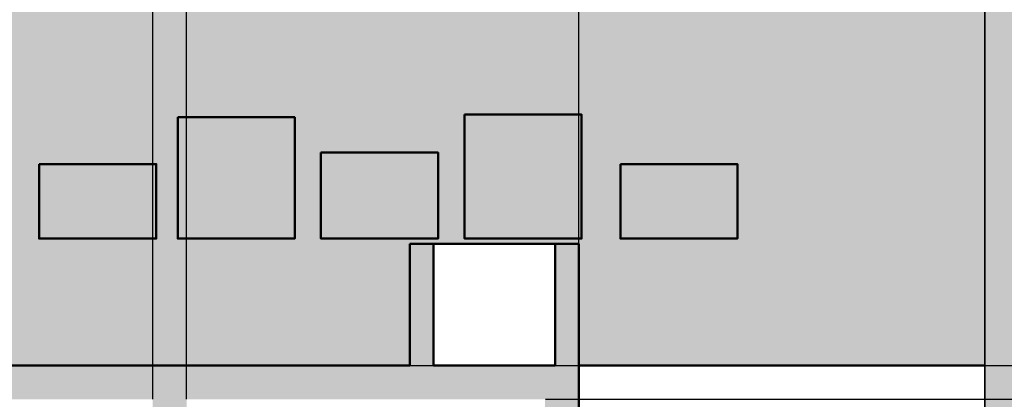
# Model space of a CAD drawing. Units: inches. Extents: x 925 to 2834, y 111 to 1355.
# Tile 21 of 25: x 1553 to 1844, y 1072 to 1184. Entities that reach past the tile are written whole.
import ezdxf

# ---------------------------------------------------------------- set-up
doc = ezdxf.new("R2010")
doc.units = ezdxf.units.IN
doc.header["$MEASUREMENT"] = 0
for name, color, linetype, lineweight in [('A-ANNO-DIMS', 2, 'Continuous', 18), ('A-ANNO-TTLB', 7, 'Continuous', 35), ('A-FLOR-PATT', 252, 'Continuous', 13), ('A-GLAZ', 3, 'Continuous', 25), ('A-WALL', 7, 'Continuous', 50)]:
    doc.layers.add(name, color=color, linetype=linetype, lineweight=lineweight)
doc.styles.get("Standard").update_dxf_attribs({"font": 'arial.ttf'})
doc.dimstyles.get("Standard").update_dxf_attribs({"dimtxt": 6, "dimasz": 3, "dimexe": 0.18, "dimexo": 0.0625, "dimgap": 0.09, "dimtad": 0, "dimtih": 1, "dimtoh": 1, "dimdec": 1, "dimzin": 0, "dimdsep": 46, "dimlunit": 3, "dimtxsty": 'Standard', "dimblk": 'ARCHTICK', "dimcen": 0.09, "dimadec": 0, "dimazin": 0, "dimtfac": 1, "dimtdec": 1, "dimtofl": 0, "dimtmove": 0, "dimatfit": 3, "dimfxl": 1, "dimtolj": 1, "dimtzin": 0, "dimarcsym": 0})

# ---------------------------------------------------------------- blocks, each defined once
blk = doc.blocks.new('_ArchTick')
at = {"color": 0, "linetype": 'ByBlock', "const_width": 0.15}
blk.add_lwpolyline([(-0.5, -0.5), (0.5, 0.5)], dxfattribs=at)
blk = doc.blocks.new('*D16')
at = {"layer": 'A-ANNO-DIMS', "color": 0, "lineweight": -2, "transparency": 16777216}
for p, q in [((1256.67, 1081.65), (1256.67, 1351.49)), ((1256.67, 1351.31), (1412.16, 1351.31)), ((1592.71, 1351.31), (1437.22, 1351.31)), ((1592.71, 1071.65), (1592.71, 1351.49))]:
    blk.add_line(p, q, dxfattribs=at)
at = {"layer": 'Defpoints', "color": 0, "transparency": 16777216}
for p in [(1592.71, 1351.31), (1256.67, 1081.59), (1592.71, 1071.59)]:
    blk.add_point(p, dxfattribs=at)
at = {"layer": 'A-ANNO-DIMS', "color": 0, "lineweight": -2, "transparency": 16777216, "xscale": 3, "yscale": 3, "zscale": 3, "rotation": 180}
blk.add_blockref('_ArchTick', (1256.67, 1351.31), dxfattribs=at)
at = {"layer": 'A-ANNO-DIMS', "color": 0, "lineweight": -2, "transparency": 16777216, "xscale": 3, "yscale": 3, "zscale": 3}
blk.add_blockref('_ArchTick', (1592.71, 1351.31), dxfattribs=at)
at = {"layer": 'A-ANNO-DIMS', "color": 0, "transparency": 16777216, "insert": (1424.69, 1351.31), "char_height": 6, "attachment_point": 5}
blk.add_mtext('\\A1;336.04', dxfattribs=at)
blk = doc.blocks.new('*D17')
at = {"layer": 'A-ANNO-DIMS', "color": 0, "lineweight": -2, "transparency": 16777216}
for p, q in [((1592.71, 1071.65), (1592.71, 1351.49)), ((1592.71, 1351.31), (1593.62, 1351.31)), ((1602.71, 1351.31), (1601.81, 1351.31)), ((1602.71, 1071.65), (1602.71, 1351.49))]:
    blk.add_line(p, q, dxfattribs=at)
at = {"layer": 'Defpoints', "color": 0, "transparency": 16777216}
for p in [(1602.71, 1351.31), (1592.71, 1071.59), (1602.71, 1071.59)]:
    blk.add_point(p, dxfattribs=at)
at = {"layer": 'A-ANNO-DIMS', "color": 0, "lineweight": -2, "transparency": 16777216, "xscale": 3, "yscale": 3, "zscale": 3, "rotation": 180}
blk.add_blockref('_ArchTick', (1592.71, 1351.31), dxfattribs=at)
at = {"layer": 'A-ANNO-DIMS', "color": 0, "lineweight": -2, "transparency": 16777216, "xscale": 3, "yscale": 3, "zscale": 3}
blk.add_blockref('_ArchTick', (1602.71, 1351.31), dxfattribs=at)
at = {"layer": 'A-ANNO-DIMS', "color": 0, "transparency": 16777216, "insert": (1597.71, 1351.31), "char_height": 6, "attachment_point": 5}
blk.add_mtext('\\A1;10', dxfattribs=at)
blk = doc.blocks.new('*D18')
at = {"layer": 'A-ANNO-DIMS', "color": 0, "lineweight": -2, "transparency": 16777216}
for p, q in [((1602.71, 1071.65), (1602.71, 1351.49)), ((1602.71, 1351.31), (1654.28, 1351.31)), ((1718.71, 1351.31), (1667.15, 1351.31)), ((1718.71, 1081.65), (1718.71, 1351.49))]:
    blk.add_line(p, q, dxfattribs=at)
at = {"layer": 'Defpoints', "color": 0, "transparency": 16777216}
for p in [(1718.71, 1351.31), (1718.71, 1081.59), (1602.71, 1071.59)]:
    blk.add_point(p, dxfattribs=at)
at = {"layer": 'A-ANNO-DIMS', "color": 0, "lineweight": -2, "transparency": 16777216, "xscale": 3, "yscale": 3, "zscale": 3, "rotation": 180}
blk.add_blockref('_ArchTick', (1602.71, 1351.31), dxfattribs=at)
at = {"layer": 'A-ANNO-DIMS', "color": 0, "lineweight": -2, "transparency": 16777216, "xscale": 3, "yscale": 3, "zscale": 3}
blk.add_blockref('_ArchTick', (1718.71, 1351.31), dxfattribs=at)
at = {"layer": 'A-ANNO-DIMS', "color": 0, "transparency": 16777216, "insert": (1660.71, 1351.31), "char_height": 6, "attachment_point": 5}
blk.add_mtext('\\A1;116', dxfattribs=at)
blk = doc.blocks.new('*D19')
at = {"layer": 'A-ANNO-DIMS', "color": 0, "lineweight": -2, "transparency": 16777216}
for p, q in [((1718.71, 1081.65), (1718.71, 1351.49)), ((1718.71, 1351.31), (1772.29, 1351.31)), ((1838.71, 1351.31), (1785.14, 1351.31)), ((1838.71, 1201.65), (1838.71, 1351.49))]:
    blk.add_line(p, q, dxfattribs=at)
at = {"layer": 'Defpoints', "color": 0, "transparency": 16777216}
for p in [(1838.71, 1351.31), (1838.71, 1201.59), (1718.71, 1081.59)]:
    blk.add_point(p, dxfattribs=at)
at = {"layer": 'A-ANNO-DIMS', "color": 0, "lineweight": -2, "transparency": 16777216, "xscale": 3, "yscale": 3, "zscale": 3, "rotation": 180}
blk.add_blockref('_ArchTick', (1718.71, 1351.31), dxfattribs=at)
at = {"layer": 'A-ANNO-DIMS', "color": 0, "lineweight": -2, "transparency": 16777216, "xscale": 3, "yscale": 3, "zscale": 3}
blk.add_blockref('_ArchTick', (1838.71, 1351.31), dxfattribs=at)
at = {"layer": 'A-ANNO-DIMS', "color": 0, "transparency": 16777216, "insert": (1778.71, 1351.31), "char_height": 6, "attachment_point": 5}
blk.add_mtext('\\A1;120', dxfattribs=at)
blk = doc.blocks.new('*D49')
at = {"layer": 'A-ANNO-DIMS', "color": 0, "lineweight": -2, "transparency": 16777216}
for p, q in [((1708.78, 1071.59), (1988.62, 1071.59)), ((1988.44, 1071.59), (1988.44, 1026.74)), ((1988.44, 975.59), (1988.44, 1020.44)), ((1708.78, 975.59), (1988.62, 975.59))]:
    blk.add_line(p, q, dxfattribs=at)
at = {"layer": 'Defpoints', "color": 0, "transparency": 16777216}
for p in [(1708.71, 1071.59), (1988.44, 1071.59), (1708.71, 975.59)]:
    blk.add_point(p, dxfattribs=at)
at = {"layer": 'A-ANNO-DIMS', "color": 0, "lineweight": -2, "transparency": 16777216, "xscale": 3, "yscale": 3, "zscale": 3}
for p, rotation in [((1988.44, 1071.59), 90), ((1988.44, 975.59), 270)]:
    blk.add_blockref('_ArchTick', p, dxfattribs=dict(at, rotation=rotation))
at = {"layer": 'A-ANNO-DIMS', "color": 0, "transparency": 16777216, "insert": (1988.44, 1023.59), "char_height": 6, "attachment_point": 5}
blk.add_mtext('\\A1;96', dxfattribs=at)
blk = doc.blocks.new('*D50')
at = {"layer": 'A-ANNO-DIMS', "color": 0, "lineweight": -2, "transparency": 16777216}
for p, q in [((1718.78, 1081.59), (1988.62, 1081.59)), ((1988.44, 1081.59), (1988.44, 1079.74)), ((1708.78, 1071.59), (1988.62, 1071.59)), ((1988.44, 1071.59), (1988.44, 1073.44))]:
    blk.add_line(p, q, dxfattribs=at)
at = {"layer": 'Defpoints', "color": 0, "transparency": 16777216}
for p in [(1718.71, 1081.59), (1988.44, 1081.59), (1708.71, 1071.59)]:
    blk.add_point(p, dxfattribs=at)
at = {"layer": 'A-ANNO-DIMS', "color": 0, "lineweight": -2, "transparency": 16777216, "xscale": 3, "yscale": 3, "zscale": 3}
for p, rotation in [((1988.44, 1081.59), 90), ((1988.44, 1071.59), 270)]:
    blk.add_blockref('_ArchTick', p, dxfattribs=dict(at, rotation=rotation))
at = {"layer": 'A-ANNO-DIMS', "color": 0, "transparency": 16777216, "insert": (1988.44, 1076.59), "char_height": 6, "attachment_point": 5}
blk.add_mtext('\\A1;10', dxfattribs=at)
blk = doc.blocks.new('*D51')
at = {"layer": 'A-ANNO-DIMS', "color": 0, "lineweight": -2, "transparency": 16777216}
for p, q in [((1838.78, 1201.59), (1988.62, 1201.59)), ((1988.44, 1201.59), (1988.44, 1144.74)), ((1988.44, 1081.59), (1988.44, 1138.44)), ((1718.78, 1081.59), (1988.62, 1081.59))]:
    blk.add_line(p, q, dxfattribs=at)
at = {"layer": 'Defpoints', "color": 0, "transparency": 16777216}
for p in [(1838.71, 1201.59), (1988.44, 1201.59), (1718.71, 1081.59)]:
    blk.add_point(p, dxfattribs=at)
at = {"layer": 'A-ANNO-DIMS', "color": 0, "lineweight": -2, "transparency": 16777216, "xscale": 3, "yscale": 3, "zscale": 3}
for p, rotation in [((1988.44, 1201.59), 90), ((1988.44, 1081.59), 270)]:
    blk.add_blockref('_ArchTick', p, dxfattribs=dict(at, rotation=rotation))
at = {"layer": 'A-ANNO-DIMS', "color": 0, "transparency": 16777216, "insert": (1988.44, 1141.59), "char_height": 6, "attachment_point": 5}
blk.add_mtext('\\A1;120', dxfattribs=at)

msp = doc.modelspace()

# ---------------------------------------------------------------- hatches: boundary and pattern name
at = {"layer": 'A-FLOR-PATT', "transparency": 33554605}
h = msp.add_hatch(color=256, dxfattribs=at)
h.dxf.hatch_style = 1
h.paths.add_polyline_path([(1931.688, 1294.5638), (991.7375, 1294.5638), (991.7375, 172.1134), (1931.688, 172.1134)])
h.paths.add_polyline_path([(1910.7128, 1273.5886), (1910.7128, 193.0886), (1012.7128, 193.0886), (1012.7128, 1273.5886)], flags=16)
h.paths.add_polyline_path([(1850.7128, 1213.5886), (1850.7128, 253.0886), (1072.7128, 253.0886), (1072.7128, 1213.5886)], flags=0)
h.paths.add_polyline_path([(1838.7128, 1201.5886), (1838.7128, 265.0886), (1084.7128, 265.0886), (1084.7128, 530.5886), (1084.7128, 1201.5886)], flags=0)
h.paths.add_polyline_path([(1547.6758, 1155.7396), (1547.6758, 1119.115), (1513.0687, 1119.115), (1513.0687, 1155.7396)], flags=0)
h.paths.add_polyline_path([(1600.1067, 1154.9439), (1634.7139, 1154.9439), (1634.7139, 1119.115), (1600.1067, 1119.115)], flags=0)
h.paths.add_polyline_path([(1505.2502, 1144.5358), (1505.2502, 1119.115), (1470.643, 1119.115), (1470.643, 1144.5358)], flags=0)
h.paths.add_polyline_path([(1559.1357, 1141.0962), (1593.7428, 1141.0962), (1593.7428, 1119.115), (1559.1357, 1119.115)], flags=0)
h.paths.add_polyline_path([(1462.8966, 1154.9439), (1462.8966, 1119.115), (1428.2895, 1119.115), (1428.2895, 1154.9439)], flags=0)
h.paths.add_polyline_path([(1642.4603, 1144.5358), (1677.0675, 1144.5358), (1677.0675, 1119.115), (1642.4603, 1119.115)], flags=0)
h.paths.add_polyline_path([(1422.3508, 1141.0962), (1422.3508, 1119.115), (1387.7436, 1119.115), (1387.7436, 1141.0962)], flags=0)
h.paths.add_polyline_path([(1684.8859, 1155.7396), (1719.4931, 1155.7396), (1719.4931, 1119.115), (1684.8859, 1119.115)], flags=0)
h.paths.add_polyline_path([(1718.7128, 1081.5886), (1718.7128, 1050.1249), (1715.7128, 1050.1249), (1715.7128, 1026.1249), (1715.7128, 1002.1249), (1718.7128, 1002.1249), (1730.7128, 1002.1249), (1730.7128, 998.1249), (1730.7128, 990.1249), (1730.7128, 986.1249), (1718.7128, 986.1249), (1718.7128, 893.5886), (1715.3735, 893.5886), (1715.3735, 891.5886), (1713.3735, 891.5886, 0.41421356), (1677.3735, 855.5886), (1713.3735, 855.5886), (1713.3735, 853.5886), (1715.3735, 853.5886), (1715.3735, 851.5886), (1718.7128, 851.5886), (1718.7128, 821.5865), (1734.4655, 821.5865), (1734.3735, 819.5886, -0.41421356), (1712.4415, 793.5886), (1712.4415, 791.5886), (1718.7128, 791.5886), (1718.7128, 717.5886), (1718.7128, 669.5886), (1732.7128, 669.5886), (1732.7128, 665.5886), (1732.7128, 641.5886), (1732.7128, 634.5886), (1732.7128, 610.5886), (1732.7128, 603.5886), (1718.7128, 603.5886), (1718.7128, 385.0886), (1434.2128, 385.0886), (1434.2128, 530.5886), (1410.2128, 530.5886), (1408.2128, 530.5886), (1408.2128, 532.5886, 0.41421356), (1372.2128, 568.5886), (1372.2128, 532.5886), (1370.2128, 532.5886), (1370.2128, 530.5886), (1368.2128, 530.5886), (1282.2128, 530.5886), (1210.2128, 530.5886), (1200.2128, 530.5886), (1200.2128, 542.1915), (1183.2307, 542.1915), (1183.2307, 546.1915), (1200.2128, 546.1915), (1200.2128, 572.1915), (1183.2307, 572.1915), (1183.2307, 576.1915), (1200.2128, 576.1915), (1200.2128, 727.5886), (1210.2128, 727.5886), (1234.2128, 727.5886), (1259.7128, 727.5886), (1259.7128, 775.5886), (1259.7128, 799.5886), (1259.7128, 847.5886), (1259.7128, 993.5872), (1259.7128, 1065.5872), (1259.7128, 1071.5886), (1219.6318, 1071.5886), (1219.6318, 1081.5886), (1084.7128, 1081.5886), (1084.7128, 1119.115), (1256.8974, 1119.115), (1256.8974, 1154.9439), (1291.5046, 1154.9439), (1291.5046, 1119.115), (1256.8974, 1119.115), (1256.6723, 1081.5886), (1293.7128, 1081.5886), (1341.7128, 1081.5886), (1341.7128, 1093.5886), (1347.7128, 1093.5886), (1371.7128, 1093.5886), (1377.7128, 1093.5886), (1377.7128, 1081.5886), (1668.7128, 1081.5886), (1668.7128, 1117.5886), (1675.7128, 1117.5886), (1711.7128, 1117.5886), (1718.7128, 1117.5886)], flags=0)
h.paths.add_polyline_path([(1376.2838, 1155.7396), (1376.2838, 1119.115), (1341.6766, 1119.115), (1341.6766, 1155.7396)], flags=0)
h.paths.add_polyline_path([(1341.7128, 1076.0886), (1293.7128, 1076.0886), (1293.7128, 1071.5886), (1269.7128, 1071.5886), (1269.7128, 1065.5872), (1266.7128, 1065.5872), (1266.7128, 1029.5872), (1265.7128, 1029.5872), (1265.7128, 993.5872), (1269.7128, 993.5872), (1269.7128, 903.5886), (1269.7128, 893.5886), (1269.7128, 847.5886), (1265.2128, 847.5886), (1265.2128, 799.5886), (1269.7128, 799.5886), (1269.7128, 775.5886), (1265.2128, 775.5886), (1265.2128, 727.5886), (1269.7128, 727.5886), (1444.2128, 727.5886), (1444.2128, 717.5886), (1234.2128, 717.5886), (1234.2128, 722.0886), (1210.2128, 722.0886), (1210.2128, 717.5886), (1210.2128, 540.5886), (1210.2128, 536.0886), (1282.2128, 536.0886), (1282.2128, 535.0886), (1210.2128, 535.0886), (1210.2128, 540.5886), (1210.2128, 717.5886), (1210.2128, 723.0886), (1234.2128, 723.0886), (1234.2128, 717.5886), (1444.2128, 717.5886), (1444.2128, 727.5886), (1269.7128, 727.5886), (1264.2128, 727.5886), (1264.2128, 775.5886), (1269.7128, 775.5886), (1269.7128, 799.5886), (1264.2128, 799.5886), (1264.2128, 847.5886), (1269.7128, 847.5886), (1269.7128, 893.5886), (1269.7128, 903.5886), (1269.7128, 993.5872), (1264.7128, 993.5872), (1264.7128, 1029.5872), (1265.7128, 1029.5872), (1265.7128, 1065.5872), (1269.7128, 1065.5872), (1269.7128, 1071.5886), (1293.7128, 1071.5886), (1293.7128, 1077.0886), (1341.7128, 1077.0886)], flags=0)
h.paths.add_polyline_path([(1730.9529, 1141.0962), (1765.5601, 1141.0962), (1765.5601, 1119.115), (1730.9529, 1119.115)], flags=0)
h.paths.add_polyline_path([(1333.8582, 1144.5358), (1333.8582, 1119.115), (1299.251, 1119.115), (1299.251, 1144.5358)], flags=0)
h.paths.add_polyline_path([(1592.7128, 968.5886), (1596.0342, 968.5886), (1602.7128, 968.5886), (1708.7128, 968.5886), (1708.7128, 903.5886), (1602.7128, 903.5886), (1602.7128, 938.5886), (1592.7128, 938.5886), (1592.7128, 903.5886), (1451.7128, 903.5886), (1451.7128, 893.5886), (1511.7128, 893.5886), (1511.7128, 881.5886), (1515.2128, 881.5886), (1518.7128, 881.5886), (1518.7128, 893.5886), (1592.7128, 893.5886), (1592.7128, 799.5886), (1518.7128, 799.5886), (1518.7128, 857.5886), (1511.7128, 857.5886), (1511.7128, 799.5886), (1511.7128, 772.0886), (1521.7128, 772.0886), (1521.7128, 792.5886), (1592.7128, 792.5886), (1592.7128, 727.5886), (1521.7128, 727.5886), (1521.7128, 748.0886), (1511.7128, 748.0886), (1511.7128, 717.5886), (1708.7128, 717.5886), (1714.2128, 717.5886), (1714.2128, 669.5886), (1708.7128, 669.5886), (1708.7128, 641.5886), (1492.2128, 641.5886), (1492.2128, 631.5886), (1621.2128, 631.5886), (1621.2128, 443.0886), (1625.7128, 443.0886), (1625.7128, 503.0886), (1625.7128, 507.5886), (1625.7128, 631.5886), (1708.7128, 631.5886), (1708.7128, 507.5886), (1655.7128, 507.5886), (1655.7128, 503.0886), (1708.7128, 503.0886), (1708.7128, 395.0886), (1625.7128, 395.0886), (1625.7128, 419.0886), (1621.2128, 419.0886), (1621.2128, 395.0886), (1482.2128, 395.0886), (1482.2128, 385.0886), (1434.2128, 385.0886), (1434.2128, 433.0886), (1444.2128, 433.0886), (1444.2128, 631.5886), (1450.2128, 631.5886), (1450.2128, 634.91), (1452.2128, 634.91), (1452.2128, 669.5886), (1454.2128, 669.5886, -0.40021217), (1490.1712, 635.3173), (1492.2128, 635.3173), (1492.2128, 641.5886), (1564.7128, 641.5886), (1564.7128, 677.5886), (1672.7128, 677.5886), (1672.7128, 681.5886), (1564.7128, 681.5886), (1564.7128, 717.5886), (1511.7128, 717.5886), (1511.7128, 748.0886), (1511.7128, 772.0886), (1511.7128, 799.5886), (1511.7128, 857.5886), (1511.8913, 857.5886), (1511.8913, 859.5886), (1515.6201, 859.5886, 0.41421356), (1537.552, 879.5886), (1513.552, 879.5886), (1511.8913, 879.5886), (1511.8913, 881.5886), (1511.7128, 881.5886), (1511.7128, 893.5886), (1451.7128, 893.5886), (1451.7128, 903.5886), (1592.7128, 903.5886), (1592.7128, 938.5886), (1592.7128, 940.5886), (1596.4415, 940.5886, 0.41421356), (1618.3735, 966.5886), (1594.3735, 966.5886), (1592.7128, 966.5886)], flags=0)
h.paths.add_polyline_path([(1377.7128, 903.5886), (1377.7128, 893.5886), (1305.7128, 893.5886), (1305.7128, 903.5886)], flags=0)
h.paths.add_polyline_path([(1708.7128, 821.5886), (1712.0342, 821.5886), (1712.0342, 819.5886), (1710.3735, 819.5886), (1708.7128, 819.5886)], flags=0)
h.paths.add_polyline_path([(1576.7128, 695.1992), (1575.5896, 693.6649), (1575.9687, 694.6994), (1575.4438, 695.1992), (1575.9687, 695.699), (1575.5896, 696.7335)], flags=0)
h.paths.add_polyline_path([(1565.9817, 662.3134), (1565.4568, 661.8136), (1565.8359, 660.7791), (1564.7128, 662.3134), (1565.8359, 663.8477), (1565.4568, 662.8132)], flags=0)
h.paths.add_polyline_path([(1444.2128, 433.0886), (1444.2128, 395.0886), (1482.2128, 395.0886), (1482.2128, 389.0886), (1438.2128, 389.0886), (1438.2128, 391.8608), (1438.2128, 433.0886)], flags=0)
h.paths.add_polyline_path([(1410.2128, 506.5886), (1410.2128, 289.0886), (1108.7128, 289.0886), (1108.7128, 506.5886)], flags=0)
h.paths.add_polyline_path([(1612.3153, 838.3016), (1680.4151, 838.3016), (1680.4151, 851.3131), (1612.3153, 851.3131)], flags=8)
h.paths.add_polyline_path([(1208.3174, 395.0436), (1282.1017, 395.0436), (1282.1017, 408.0552), (1208.3174, 408.0552)], flags=8)
h.paths.add_polyline_path([(1291.8049, 598.7427), (1369.8017, 598.7427), (1369.8017, 611.7542), (1291.8049, 611.7542)], flags=8)
h.paths.add_polyline_path([(1119.679, 917.3022), (1191.0817, 917.3022), (1191.0817, 930.3137), (1119.679, 930.3137)], flags=8)
h.paths.add_polyline_path([(1332.2261, 815.9808), (1410.2258, 815.9808), (1410.2258, 829.001), (1332.2261, 829.001)], flags=8)
h.paths.add_polyline_path([(1390.9013, 955.8158), (1475.4981, 955.8158), (1475.4981, 968.8273), (1390.9013, 968.8273)], flags=8)
h.paths.add_polyline_path([(1620.3436, 998.9325), (1688.4434, 998.9325), (1688.4434, 1011.944), (1620.3436, 1011.944)], flags=8)
h.paths.add_polyline_path([(1620.3436, 914.1039), (1691.7405, 914.1039), (1691.7405, 927.1155), (1620.3436, 927.1155)], flags=8)
h.paths.add_polyline_path([(1521.4542, 816.005), (1589.5569, 816.005), (1589.5569, 829.0253), (1521.4542, 829.0253)], flags=8)
h.paths.add_polyline_path([(1528.524, 740.3497), (1602.3082, 740.3497), (1602.3082, 753.3613), (1528.524, 753.3613)], flags=8)
h.paths.add_polyline_path([(1627.6094, 762.6128), (1702.3091, 762.6128), (1702.3091, 775.6244), (1627.6094, 775.6244)], flags=8)
h.paths.add_polyline_path([(1610.5442, 657.2751), (1684.3284, 657.2751), (1684.3284, 670.2867), (1610.5442, 670.2867)], flags=8)
h.paths.add_polyline_path([(1636.6983, 519.472), (1711.3981, 519.472), (1711.3981, 532.4835), (1636.6983, 532.4835)], flags=8)
h.paths.add_polyline_path([(1616.8577, 424.8539), (1694.8545, 424.8539), (1694.8545, 437.8654), (1616.8577, 437.8654)], flags=8)
h.paths.add_polyline_path([(1506.1456, 460.8838), (1579.9299, 460.8838), (1579.9299, 473.8953), (1506.1456, 473.8953)], flags=8)
h.paths.add_polyline_path([(1624.6119, 784.6011), (1696.9185, 784.6011), (1696.9185, 797.7864), (1624.6119, 797.7864)], flags=8)
h.paths.add_polyline_path([(1606.3732, 854.2194), (1683.3039, 854.2194), (1683.3039, 867.4048), (1606.3732, 867.4048)], flags=8)
h.paths.add_polyline_path([(1127.8008, 940.3581), (1165.1637, 940.3581), (1165.1637, 953.5348), (1127.8008, 953.5348)], flags=8)
h.paths.add_polyline_path([(1620.8657, 1019.4968), (1677.3447, 1019.4968), (1677.3447, 1032.6735), (1620.8657, 1032.6735)], flags=8)
h.paths.add_polyline_path([(1620.8643, 930.1821), (1703.0564, 930.1821), (1703.0564, 943.3675), (1620.8643, 943.3675)], flags=8)
h.paths.add_polyline_path([(1324.5702, 836.8338), (1408.0892, 836.8338), (1408.0892, 850.0191), (1324.5702, 850.0191)], flags=8)
h.paths.add_polyline_path([(1281.6584, 622.8885), (1383.6213, 622.8885), (1383.6213, 636.0739), (1281.6584, 636.0739)], flags=8)
h.paths.add_polyline_path([(1210.6721, 416.7893), (1269.1299, 416.7893), (1269.1299, 429.9747), (1210.6721, 429.9747)], flags=8)
h.paths.add_polyline_path([(1507.8264, 477.4836), (1586.7329, 477.4836), (1586.7329, 490.669), (1507.8264, 490.669)], flags=8)
h.paths.add_polyline_path([(1643.6238, 443.8135), (1696.6696, 443.8135), (1696.6696, 456.5643), (1643.6238, 456.5643)], flags=8)
h.paths.add_polyline_path([(1647.2466, 540.5638), (1693.1825, 540.5638), (1693.1825, 553.7491), (1647.2466, 553.7491)], flags=8)
h.paths.add_polyline_path([(1626.0633, 668.5064), (1673.3174, 668.5064), (1673.3174, 681.6831), (1626.0633, 681.6831)], flags=8)
h.paths.add_polyline_path([(1538.2915, 830.7872), (1567.5942, 830.7872), (1567.5942, 843.5293), (1538.2915, 843.5293)], flags=8)
h.paths.add_polyline_path([(1530.9338, 754.0477), (1559.576, 754.0477), (1559.576, 766.7898), (1530.9338, 766.7898)], flags=8)
h.paths.add_polyline_path([(1351.2461, 979.2309), (1513.8919, 979.2309), (1513.8919, 992.4076), (1351.2461, 992.4076)], flags=8)
at = {"layer": 'A-FLOR-PATT'}
h = msp.add_hatch(color=256, dxfattribs=at)
h.dxf.hatch_style = 1
h.paths.add_polyline_path([(1850.7128, 1213.5886), (1072.7128, 1213.5886), (1072.7128, 253.0886), (1850.7128, 253.0886)])
h.paths.add_polyline_path([(1084.7128, 1201.5886), (1838.7128, 1201.5886), (1838.7128, 265.0886), (1084.7128, 265.0886)], flags=16)
h.paths.add_polyline_path([(1183.2307, 576.1915), (1200.2128, 576.1915), (1200.2128, 727.5886), (1210.2128, 727.5886), (1234.2128, 727.5886), (1259.7128, 727.5886), (1259.7128, 775.5886), (1259.7128, 799.5886), (1259.7128, 847.5886), (1259.7128, 993.5872), (1259.7128, 1065.5872), (1259.7128, 1071.5886), (1219.6318, 1071.5886), (1219.6318, 1081.5886), (1293.7128, 1081.5886), (1341.7128, 1081.5886), (1341.7128, 1093.5886), (1347.7128, 1093.5886), (1347.7128, 1081.5886), (1371.7128, 1081.5886), (1371.7128, 1093.5886), (1377.7128, 1093.5886), (1377.7128, 1081.5886), (1668.7128, 1081.5886), (1668.7128, 1117.5886), (1675.7128, 1117.5886), (1675.7128, 1081.5886), (1711.7128, 1081.5886), (1711.7128, 1117.5886), (1718.7128, 1117.5886), (1718.7128, 1081.5886), (1718.7128, 1050.1249), (1715.7128, 1050.1249), (1715.7128, 1026.1249), (1715.7128, 1002.1249), (1718.7128, 1002.1249), (1730.7128, 1002.1249), (1730.7128, 998.1249), (1730.7128, 990.1249), (1730.7128, 986.1249), (1718.7128, 986.1249), (1718.7128, 893.5886), (1715.3735, 893.5886), (1715.3735, 891.5886), (1713.3735, 891.5886, 0.41421356), (1677.3735, 855.5886), (1713.3735, 855.5886), (1713.3735, 853.5886), (1715.3735, 853.5886), (1715.3735, 851.5886), (1718.7128, 851.5886), (1718.7128, 821.5865), (1734.4655, 821.5865), (1734.3735, 819.5886, -0.41421356), (1712.4415, 793.5886), (1712.4415, 791.5886), (1718.7128, 791.5886), (1718.7128, 717.5886), (1718.7128, 669.5886), (1732.7128, 669.5886), (1732.7128, 665.5886), (1732.7128, 641.5886), (1732.7128, 634.5886), (1732.7128, 610.5886), (1732.7128, 603.5886), (1718.7128, 603.5886), (1718.7128, 385.0886), (1434.2128, 385.0886), (1434.2128, 433.0886), (1434.2128, 530.5886), (1410.2128, 530.5886), (1408.2128, 530.5886), (1408.2128, 532.5886, 0.41421356), (1372.2128, 568.5886), (1372.2128, 532.5886), (1370.2128, 532.5886), (1370.2128, 530.5886), (1368.2128, 530.5886), (1282.2128, 530.5886), (1210.2128, 530.5886), (1200.2128, 530.5886), (1200.2128, 542.1915), (1183.2307, 542.1915), (1183.2307, 546.1915), (1200.2128, 546.1915), (1200.2128, 572.1915), (1183.2307, 572.1915)], flags=0)
h.paths.add_polyline_path([(1210.2128, 717.5886), (1210.2128, 723.0886), (1234.2128, 723.0886), (1234.2128, 717.5886), (1444.2128, 717.5886), (1444.2128, 727.5886), (1269.7128, 727.5886), (1264.2128, 727.5886), (1264.2128, 775.5886), (1269.7128, 775.5886), (1269.7128, 799.5886), (1264.2128, 799.5886), (1264.2128, 847.5886), (1269.7128, 847.5886), (1269.7128, 893.5886), (1269.7128, 903.5886), (1269.7128, 993.5872), (1264.7128, 993.5872), (1264.7128, 1029.5872), (1265.7128, 1029.5872), (1265.7128, 1065.5872), (1269.7128, 1065.5872), (1269.7128, 1071.5886), (1293.7128, 1071.5886), (1293.7128, 1077.0886), (1341.7128, 1077.0886), (1341.7128, 1076.0886), (1293.7128, 1076.0886), (1293.7128, 1071.5886), (1269.7128, 1071.5886), (1269.7128, 1065.5872), (1266.7128, 1065.5872), (1266.7128, 1029.5872), (1265.7128, 1029.5872), (1265.7128, 993.5872), (1269.7128, 993.5872), (1269.7128, 903.5886), (1269.7128, 893.5886), (1269.7128, 847.5886), (1265.2128, 847.5886), (1265.2128, 799.5886), (1269.7128, 799.5886), (1269.7128, 775.5886), (1265.2128, 775.5886), (1265.2128, 727.5886), (1269.7128, 727.5886), (1444.2128, 727.5886), (1444.2128, 717.5886), (1234.2128, 717.5886), (1234.2128, 722.0886), (1210.2128, 722.0886), (1210.2128, 717.5886), (1210.2128, 540.5886), (1210.2128, 536.0886), (1282.2128, 536.0886), (1282.2128, 535.0886), (1210.2128, 535.0886), (1210.2128, 540.5886)], flags=0)
h.paths.add_polyline_path([(1450.2128, 634.91), (1452.2128, 634.91), (1452.2128, 669.5886), (1454.2128, 669.5886, -0.40021217), (1490.1712, 635.3173), (1492.2128, 635.3173), (1492.2128, 641.5886), (1564.7128, 641.5886), (1564.7128, 677.5886), (1672.7128, 677.5886), (1672.7128, 681.5886), (1564.7128, 681.5886), (1564.7128, 717.5886), (1511.7128, 717.5886), (1511.7128, 748.0886), (1511.7128, 772.0886), (1511.7128, 799.5886), (1511.7128, 857.5886), (1511.8913, 857.5886), (1511.8913, 859.5886), (1515.6201, 859.5886, 0.41421356), (1537.552, 879.5886), (1513.552, 879.5886), (1511.8913, 879.5886), (1511.8913, 881.5886), (1511.7128, 881.5886), (1511.7128, 893.5886), (1451.7128, 893.5886), (1451.7128, 903.5886), (1592.7128, 903.5886), (1592.7128, 938.5886), (1592.7128, 940.5886), (1596.4415, 940.5886, 0.41421356), (1618.3735, 966.5886), (1594.3735, 966.5886), (1592.7128, 966.5886), (1592.7128, 968.5886), (1596.0342, 968.5886), (1602.7128, 968.5886), (1708.7128, 968.5886), (1708.7128, 903.5886), (1602.7128, 903.5886), (1602.7128, 938.5886), (1592.7128, 938.5886), (1592.7128, 903.5886), (1451.7128, 903.5886), (1451.7128, 893.5886), (1511.7128, 893.5886), (1511.7128, 881.5886), (1518.7128, 881.5886), (1518.7128, 893.5886), (1592.7128, 893.5886), (1592.7128, 799.5886), (1518.7128, 799.5886), (1518.7128, 857.5886), (1511.7128, 857.5886), (1511.7128, 799.5886), (1511.7128, 772.0886), (1521.7128, 772.0886), (1521.7128, 792.5886), (1592.7128, 792.5886), (1592.7128, 727.5886), (1521.7128, 727.5886), (1521.7128, 748.0886), (1511.7128, 748.0886), (1511.7128, 717.5886), (1708.7128, 717.5886), (1714.2128, 717.5886), (1714.2128, 669.5886), (1708.7128, 669.5886), (1708.7128, 641.5886), (1492.2128, 641.5886), (1492.2128, 631.5886), (1621.2128, 631.5886), (1621.2128, 443.0886), (1625.7128, 443.0886), (1625.7128, 503.0886), (1625.7128, 507.5886), (1625.7128, 631.5886), (1708.7128, 631.5886), (1708.7128, 507.5886), (1655.7128, 507.5886), (1655.7128, 503.0886), (1708.7128, 503.0886), (1708.7128, 395.0886), (1625.7128, 395.0886), (1625.7128, 419.0886), (1621.2128, 419.0886), (1621.2128, 395.0886), (1482.2128, 395.0886), (1482.2128, 389.0886), (1438.2128, 389.0886), (1438.2128, 391.8608), (1438.2128, 433.0886), (1444.2128, 433.0886), (1444.2128, 631.5886), (1450.2128, 631.5886)], flags=0)
h.paths.add_polyline_path([(1444.2128, 433.0886), (1444.2128, 395.0886), (1482.2128, 395.0886), (1482.2128, 391.0886), (1440.2128, 391.0886), (1440.2128, 391.8608), (1440.2128, 433.0886)], flags=0)
h.paths.add_polyline_path([(1305.7128, 893.5886), (1305.7128, 903.5886), (1377.7128, 903.5886), (1377.7128, 893.5886)], flags=0)
h.paths.add_polyline_path([(1564.7128, 662.3134), (1565.8359, 663.8477), (1565.4568, 662.8132), (1565.9817, 662.3134), (1565.4568, 661.8136), (1565.8359, 660.7791)], flags=0)
h.paths.add_polyline_path([(1575.4438, 695.1992), (1575.9687, 695.699), (1575.5896, 696.7335), (1576.7128, 695.1992), (1575.5896, 693.6649), (1575.9687, 694.6994)], flags=0)
h.paths.add_polyline_path([(1708.7128, 821.5886), (1712.0342, 821.5886), (1712.0342, 819.5886), (1710.3735, 819.5886), (1708.7128, 819.5886)], flags=0)
at = {"layer": 'A-FLOR-PATT', "transparency": 33554554}
h = msp.add_hatch(color=256, dxfattribs=at)
h.dxf.hatch_style = 1
h.paths.add_polyline_path([(1838.7128, 1201.5886), (1084.7128, 1201.5886), (1084.7128, 1119.115), (1256.8974, 1119.115), (1256.8974, 1154.9439), (1291.5046, 1154.9439), (1291.5046, 1119.115), (1256.8974, 1119.115), (1256.6723, 1081.5886), (1293.7128, 1081.5886), (1341.7128, 1081.5886), (1341.7128, 1093.5886), (1347.7128, 1093.5886), (1371.7128, 1093.5886), (1377.7128, 1093.5886), (1377.7128, 1081.5886), (1668.7128, 1081.5886), (1668.7128, 1117.5886), (1675.7128, 1117.5886), (1711.7128, 1117.5886), (1718.7128, 1117.5886), (1718.7128, 1081.5886), (1838.7128, 1081.5886)])
h.paths.add_polyline_path([(1299.251, 1144.5358), (1333.8582, 1144.5358), (1333.8582, 1119.115), (1299.251, 1119.115)], flags=16)
h.paths.add_polyline_path([(1341.6766, 1155.7396), (1376.2838, 1155.7396), (1376.2838, 1119.115), (1341.6766, 1119.115)], flags=16)
h.paths.add_polyline_path([(1387.7436, 1141.0962), (1422.3508, 1141.0962), (1422.3508, 1119.115), (1387.7436, 1119.115)], flags=16)
h.paths.add_polyline_path([(1428.2895, 1154.9439), (1462.8966, 1154.9439), (1462.8966, 1119.115), (1428.2895, 1119.115)], flags=16)
h.paths.add_polyline_path([(1470.643, 1144.5358), (1505.2502, 1144.5358), (1505.2502, 1119.115), (1470.643, 1119.115)], flags=16)
h.paths.add_polyline_path([(1513.0687, 1155.7396), (1547.6758, 1155.7396), (1547.6758, 1119.115), (1513.0687, 1119.115)], flags=16)
h.paths.add_polyline_path([(1559.1357, 1141.0962), (1593.7428, 1141.0962), (1593.7428, 1119.115), (1559.1357, 1119.115)], flags=16)
h.paths.add_polyline_path([(1600.1067, 1154.9439), (1634.7139, 1154.9439), (1634.7139, 1119.115), (1600.1067, 1119.115)], flags=16)
h.paths.add_polyline_path([(1642.4603, 1144.5358), (1677.0675, 1144.5358), (1677.0675, 1119.115), (1642.4603, 1119.115)], flags=16)
h.paths.add_polyline_path([(1684.8859, 1155.7396), (1719.4931, 1155.7396), (1719.4931, 1119.115), (1684.8859, 1119.115)], flags=16)
h.paths.add_polyline_path([(1730.9529, 1141.0962), (1765.5601, 1141.0962), (1765.5601, 1119.115), (1730.9529, 1119.115)], flags=16)
at = {"layer": 'A-FLOR-PATT', "transparency": 33554661}
h = msp.add_hatch(color=256, dxfattribs=at)
h.dxf.hatch_style = 1
h.paths.add_polyline_path([(1291.5046, 1154.9439), (1256.8974, 1154.9439), (1256.8974, 1119.115), (1291.5046, 1119.115)])
h.paths.add_polyline_path([(1333.8582, 1144.5358), (1299.251, 1144.5358), (1299.251, 1119.115), (1333.8582, 1119.115)])
h.paths.add_polyline_path([(1376.2838, 1155.7396), (1341.6766, 1155.7396), (1341.6766, 1119.115), (1376.2838, 1119.115)])
h.paths.add_polyline_path([(1422.3508, 1141.0962), (1387.7436, 1141.0962), (1387.7436, 1119.115), (1422.3508, 1119.115)])
h.paths.add_polyline_path([(1462.8966, 1154.9439), (1428.2895, 1154.9439), (1428.2895, 1119.115), (1462.8966, 1119.115)])
h.paths.add_polyline_path([(1505.2502, 1144.5358), (1470.643, 1144.5358), (1470.643, 1119.115), (1505.2502, 1119.115)])
h.paths.add_polyline_path([(1547.6758, 1155.7396), (1513.0687, 1155.7396), (1513.0687, 1119.115), (1547.6758, 1119.115)])
h.paths.add_polyline_path([(1593.7428, 1141.0962), (1559.1357, 1141.0962), (1559.1357, 1119.115), (1593.7428, 1119.115)])
h.paths.add_polyline_path([(1634.7139, 1154.9439), (1600.1067, 1154.9439), (1600.1067, 1119.115), (1634.7139, 1119.115)])
h.paths.add_polyline_path([(1677.0675, 1144.5358), (1642.4603, 1144.5358), (1642.4603, 1119.115), (1677.0675, 1119.115)])
h.paths.add_polyline_path([(1719.4931, 1155.7396), (1684.8859, 1155.7396), (1684.8859, 1119.115), (1719.4931, 1119.115)])
h.paths.add_polyline_path([(1765.5601, 1141.0962), (1730.9529, 1141.0962), (1730.9529, 1119.115), (1765.5601, 1119.115)])
at = {"layer": 'A-FLOR-PATT'}
h = msp.add_hatch(color=256, dxfattribs=at)
h.dxf.hatch_style = 1
h.paths.add_polyline_path([(1718.7128, 603.5886), (1708.7128, 603.5886), (1708.7128, 507.5886), (1655.7128, 507.5886), (1655.7128, 503.0886), (1708.7128, 503.0886), (1708.7128, 395.0886), (1625.7128, 395.0886), (1625.7128, 419.0886), (1621.2128, 419.0886), (1621.2128, 395.0886), (1482.2128, 395.0886), (1482.2128, 385.0886), (1718.7128, 385.0886)])
h.paths.add_polyline_path([(1625.7128, 631.5886), (1708.7128, 631.5886), (1708.7128, 603.5886), (1718.7128, 603.5886), (1732.7128, 603.5886), (1732.7128, 610.5886), (1715.7128, 610.5886), (1715.7128, 634.5886), (1732.7128, 634.5886), (1732.7128, 641.5886), (1715.7128, 641.5886), (1715.7128, 665.5886), (1732.7128, 665.5886), (1732.7128, 669.5886), (1708.7128, 669.5886), (1708.7128, 641.5886), (1492.2128, 641.5886), (1492.2128, 631.5886), (1621.2128, 631.5886), (1621.2128, 443.0886), (1625.7128, 443.0886), (1625.7128, 503.0886), (1625.7128, 507.5886)])
h.paths.add_polyline_path([(1718.7128, 851.5886), (1708.7128, 851.5886), (1708.7128, 828.5886), (1602.7128, 828.5886), (1602.7128, 893.5886), (1708.7128, 893.5886), (1718.7128, 893.5886), (1718.7128, 986.1249), (1730.7128, 986.1249), (1730.7128, 990.1249), (1718.7128, 990.1249), (1718.7128, 998.1249), (1730.7128, 998.1249), (1730.7128, 1002.1249), (1718.7128, 1002.1249), (1708.7128, 1002.1249), (1708.7128, 975.5886), (1602.7128, 975.5886), (1602.7128, 1011.5886), (1592.7128, 1011.5886), (1592.7128, 968.5886), (1596.0342, 968.5886), (1602.7128, 968.5886), (1708.7128, 968.5886), (1708.7128, 903.5886), (1602.7128, 903.5886), (1602.7128, 938.5886), (1592.7128, 938.5886), (1592.7128, 903.5886), (1451.7128, 903.5886), (1451.7128, 893.5886), (1511.7128, 893.5886), (1511.7128, 881.5886), (1515.2128, 881.5886), (1518.7128, 881.5886), (1518.7128, 893.5886), (1592.7128, 893.5886), (1592.7128, 799.5886), (1518.7128, 799.5886), (1518.7128, 857.5886), (1511.7128, 857.5886), (1511.7128, 799.5886), (1511.7128, 772.0886), (1521.7128, 772.0886), (1521.7128, 792.5886), (1592.7128, 792.5886), (1592.7128, 727.5886), (1521.7128, 727.5886), (1521.7128, 748.0886), (1511.7128, 748.0886), (1511.7128, 717.5886), (1708.7128, 717.5886), (1718.7128, 717.5886), (1718.7128, 727.5886), (1718.7128, 791.5886), (1708.7128, 791.5886), (1708.7128, 727.5886), (1602.7128, 727.5886), (1602.7128, 821.5886), (1708.7128, 821.5886), (1712.0342, 821.5886), (1718.7128, 821.5886)])
h.paths.add_polyline_path([(1718.7128, 1081.5886), (1718.7128, 1117.5886), (1711.7128, 1117.5886), (1711.7128, 1081.5886), (1675.7128, 1081.5886), (1675.7128, 1117.5886), (1668.7128, 1117.5886), (1668.7128, 1081.5886), (1377.7128, 1081.5886), (1377.7128, 1093.5886), (1371.7128, 1093.5886), (1371.7128, 1081.5886), (1347.7128, 1081.5886), (1347.7128, 1093.5886), (1341.7128, 1093.5886), (1341.7128, 1081.5886), (1341.7128, 1071.5886), (1592.7128, 1071.5886), (1592.7128, 1035.5886), (1602.7128, 1035.5886), (1602.7128, 1071.5886), (1708.7128, 1071.5886), (1708.7128, 1050.1249), (1718.7128, 1050.1249)])
h.paths.add_polyline_path([(1293.7128, 1081.5886), (1219.6318, 1081.5886), (1219.6318, 1071.5886), (1259.7128, 1071.5886), (1259.7128, 1065.5872), (1269.7128, 1065.5872), (1269.7128, 1071.5886), (1293.7128, 1071.5886)])
h.paths.add_polyline_path([(1269.7128, 903.5886), (1269.7128, 993.5872), (1259.7128, 993.5872), (1259.7128, 847.5886), (1269.7128, 847.5886), (1269.7128, 893.5886)])
h.paths.add_polyline_path([(1377.7128, 903.5886), (1305.7128, 903.5886), (1305.7128, 893.5886), (1377.7128, 893.5886)])
h.paths.add_polyline_path([(1444.2128, 727.5886), (1269.7128, 727.5886), (1259.7128, 727.5886), (1234.2128, 727.5886), (1234.2128, 717.5886), (1444.2128, 717.5886)])
h.paths.add_polyline_path([(1269.7128, 799.5886), (1259.7128, 799.5886), (1259.7128, 775.5886), (1269.7128, 775.5886)])
h.paths.add_polyline_path([(1444.2128, 631.5886), (1450.2128, 631.5886), (1450.2128, 634.91), (1450.2128, 641.5886), (1434.2128, 641.5886), (1434.2128, 540.5886), (1410.2128, 540.5886), (1410.2128, 530.5886), (1434.2128, 530.5886), (1434.2128, 433.0886), (1444.2128, 433.0886)])
h.paths.add_polyline_path([(1368.2128, 533.91), (1368.2128, 540.5886), (1282.2128, 540.5886), (1282.2128, 530.5886), (1368.2128, 530.5886)])
h.paths.add_polyline_path([(1210.2128, 717.5886), (1210.2128, 727.5886), (1200.2128, 727.5886), (1200.2128, 576.1915), (1183.2307, 576.1915), (1183.2307, 572.1915), (1200.2128, 572.1915), (1200.2128, 546.1915), (1183.2307, 546.1915), (1183.2307, 542.1915), (1200.2128, 542.1915), (1200.2128, 530.5886), (1210.2128, 530.5886), (1210.2128, 540.5886)])

# ---------------------------------------------------------------- linework, layer by layer
at = {"layer": 'A-ANNO-TTLB'}
for p, q in [((1838.7128, 1201.5886), (1838.7128, 265.0886)), ((1838.7128, 265.0886), (1838.7128, 1081.5886))]:
    msp.add_line(p, q, dxfattribs=at)
msp.add_lwpolyline([(1084.7128, 265.0886), (1838.7128, 265.0886), (1838.7128, 1201.5886), (1084.7128, 1201.5886)], close=True, dxfattribs=at)
at = {"layer": 'A-GLAZ'}
msp.add_line((1084.7128, 1081.5886), (1838.7128, 1081.5886), dxfattribs=at)
at = {"layer": 'A-WALL'}
for p, q in [((1668.7128, 1081.5886), (1668.7128, 1117.5886)), ((1668.7128, 1117.5886), (1675.7128, 1117.5886)), ((1675.7128, 1081.5886), (1675.7128, 1117.5886)), ((1675.7128, 1117.5886), (1711.7128, 1117.5886)), ((1711.7128, 1081.5886), (1711.7128, 1117.5886)), ((1711.7128, 1117.5886), (1718.7128, 1117.5886)), ((1718.7128, 1081.5886), (1718.7128, 1117.5886)), ((1377.7128, 1081.5886), (1668.7128, 1081.5886)), ((1675.7128, 1081.5886), (1711.7128, 1081.5886)), ((1718.7128, 1081.5886), (1718.7128, 1050.1249)), ((1718.7128, 1081.5886), (1838.7128, 1081.5886)), ((1838.7128, 1081.5886), (1718.7128, 1081.5886)), ((1718.7128, 1081.5886), (1718.7128, 1050.1249))]:
    msp.add_line(p, q, dxfattribs=at)
for points in [[(1684.8859, 1155.7396), (1719.4931, 1155.7396), (1719.4931, 1119.115), (1684.8859, 1119.115)], [(1600.1067, 1154.9439), (1634.7139, 1154.9439), (1634.7139, 1119.115), (1600.1067, 1119.115)], [(1642.4603, 1144.5358), (1677.0675, 1144.5358), (1677.0675, 1119.115), (1642.4603, 1119.115)], [(1559.1357, 1141.0962), (1593.7428, 1141.0962), (1593.7428, 1119.115), (1559.1357, 1119.115)], [(1730.9529, 1141.0962), (1765.5601, 1141.0962), (1765.5601, 1119.115), (1730.9529, 1119.115)]]:
    msp.add_lwpolyline(points, close=True, dxfattribs=at)

# ---------------------------------------------------------------- dimensions: what is measured, and where the dimension line sits
at = {"layer": 'A-ANNO-DIMS'}
for base, p1, p2, override, picture, middle in [((1592.7128, 1351.3138), (1256.6723, 1081.5886), (1592.7128, 1071.5886), {"dimdec": 2, "dimlfac": 1, "dimrnd": 0, "dimzin": 0, "dimdsep": 46, "dimlunit": 2}, '*D16', (1424.6925, 1351.3138)), ((1602.7128, 1351.3138), (1592.7128, 1071.5886), (1602.7128, 1071.5886), {"dimdec": 0, "dimlfac": 1, "dimrnd": 0, "dimzin": 0, "dimdsep": 46, "dimlunit": 2}, '*D17', (1597.7128, 1351.3138)), ((1718.7128, 1351.3138), (1602.7128, 1071.5886), (1718.7128, 1081.5886), {"dimdec": 0, "dimlfac": 1, "dimrnd": 0, "dimzin": 0, "dimdsep": 46, "dimlunit": 2}, '*D18', (1660.7128, 1351.3138)), ((1838.7128, 1351.3138), (1718.7128, 1081.5886), (1838.7128, 1201.5886), {"dimdec": 0, "dimlfac": 1, "dimrnd": 0, "dimzin": 0, "dimdsep": 46, "dimlunit": 2}, '*D19', (1778.7128, 1351.3138))]:
    dim = msp.add_linear_dim(base=base, p1=p1, p2=p2, dimstyle='Standard', override=override, dxfattribs=at)
    dim.commit()
    dim.dimension.update_dxf_attribs({"geometry": picture, "text_midpoint": middle})
for base, p1, p2, picture, middle in [((1988.438, 1201.5886), (1718.7128, 1081.5886), (1838.7128, 1201.5886), '*D51', (1988.438, 1141.5886)), ((1988.438, 1081.5886), (1708.7128, 1071.5886), (1718.7128, 1081.5886), '*D50', (1988.438, 1076.5886)), ((1988.438, 1071.5886), (1708.7128, 975.5886), (1708.7128, 1071.5886), '*D49', (1988.438, 1023.5886))]:
    dim = msp.add_linear_dim(base=base, p1=p1, p2=p2, angle=90, dimstyle='Standard', override={"dimdec": 0, "dimlfac": 1, "dimrnd": 0, "dimzin": 0, "dimdsep": 46, "dimlunit": 2}, dxfattribs=at)
    dim.commit()
    dim.dimension.update_dxf_attribs({"geometry": picture, "text_midpoint": middle})

doc.saveas('drawing.dxf')
